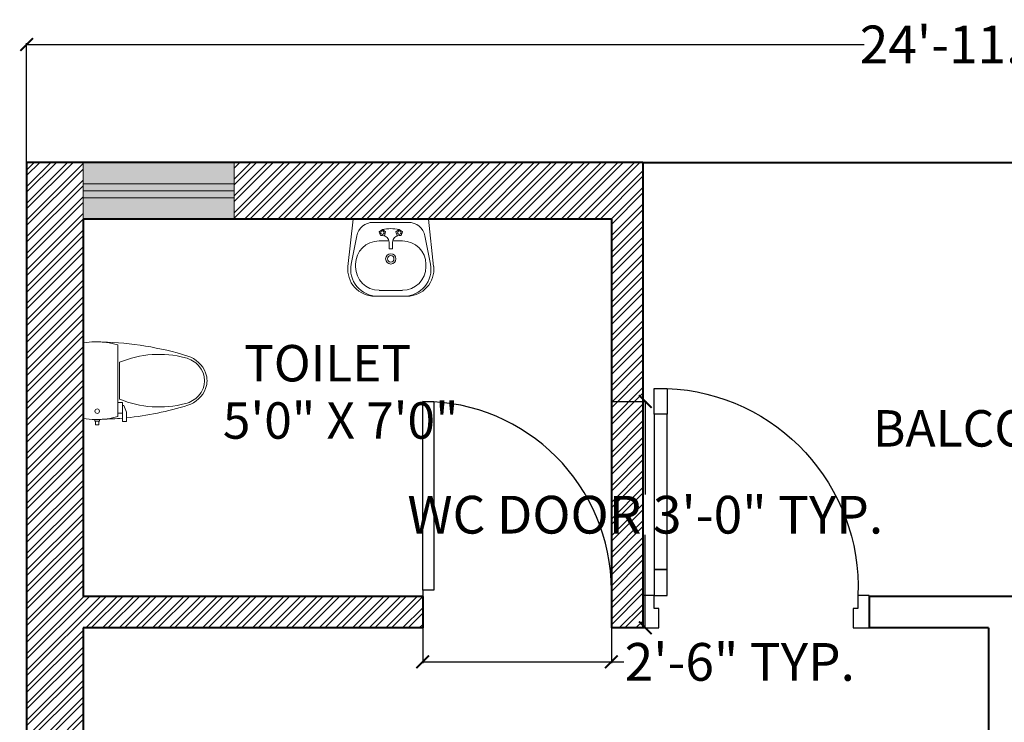
# Model space of a CAD drawing. Units: inches. Extents: x 528 to 2520, y -151 to 1354.
# Tile 20 of 41: x 1123 to 1279, y 1228 to 1340. Entities that reach past the tile are written whole.
import ezdxf

# ---------------------------------------------------------------- set-up
doc = ezdxf.new("R2010")
doc.units = ezdxf.units.IN
doc.header["$MEASUREMENT"] = 0
for name, color, linetype, lineweight in [('A-ANNO-DIMS', 2, 'Continuous', 18), ('A-AREA-IDEN', 7, 'Continuous', 18), ('A-Door', 150, 'Continuous', 25), ('A-FLOR-FIXT', 9, 'Continuous', 18), ('A-WALL-PATT', 6, 'Continuous', 13), ('walls', 7, 'Continuous', 40), ('WINDOWS', 2, 'Continuous', 20)]:
    doc.layers.add(name, color=color, linetype=linetype, lineweight=lineweight)
doc.layers.add('A-GLAZ-PATT', color=152, linetype='Continuous', lineweight=13, true_color=0x2776bb)
doc.layers.add('NT', color=1, linetype='Continuous')
doc.styles.get("Standard").update_dxf_attribs({"font": 'arial.ttf'})
doc.dimstyles.get("Standard").update_dxf_attribs({"dimtxt": 6, "dimasz": 2, "dimexe": 0.18, "dimexo": 0.0625, "dimgap": 0.09, "dimtad": 0, "dimtih": 1, "dimtoh": 1, "dimdec": 1, "dimzin": 0, "dimdsep": 46, "dimlunit": 3, "dimtxsty": 'Standard', "dimblk": 'ARCHTICK', "dimcen": 0.09, "dimadec": 0, "dimazin": 0, "dimtfac": 1, "dimtdec": 1, "dimtofl": 0, "dimtmove": 0, "dimatfit": 3, "dimfxl": 1, "dimtolj": 1, "dimtzin": 0, "dimarcsym": 0})

# ---------------------------------------------------------------- blocks, each defined once
blk = doc.blocks.new('A$C7DB75F4D')
at = {"layer": 'A-Door'}
for points in [[(625, 740), (625, 660), (665, 660), (665, 740)], [(625, 180), (625, 660), (665, 660), (665, 180)], [(625, 100), (625, 180), (665, 180), (665, 100)], [(35, 100), (35, 60), (50, 60), (50, 50), (50, 0), (0, 0), (0, 100)], [(665, 100), (700, 100), (700, 0), (650, 0), (650, 50), (650, 60), (665, 60)]]:
    blk.add_lwpolyline(points, close=True, dxfattribs=at)
at = {"layer": 'NT'}
blk.add_arc((650, 125), 615.5, 92.3278, 182.3278, dxfattribs=at)
blk = doc.blocks.new('toilet-7')
at = {"color": 0, "linetype": 'ByBlock'}
for p, q in [((0.2097, -0.02), (-0.2097, -0.02)), ((0.2151, -0.0677), (0.2097, -0.02)), ((-0.2457, -0.0874), (-0.2457, -0.1068)), ((-0.2457, -0.0874), (-0.2257, -0.0874)), ((-0.2457, -0.1068), (-0.2257, -0.1068)), ((-0.2257, -0.0846), (-0.2257, -0.1096)), ((-0.2257, -0.0846), (-0.2157, -0.0846)), ((0.2151, -0.1171), (0.2151, -0.0677)), ((-0.2257, -0.1096), (-0.2154, -0.1096)), ((0.1991, -0.2124), (0.2099, -0.164)), ((0.2099, -0.164), (0.2151, -0.1171)), ((0.1991, -0.2124), (-0.1991, -0.2124)), ((-0.1803, -0.2374), (-0.1803, -0.2124)), ((-0.1213, -0.2374), (-0.1213, -0.2124)), ((-0.1213, -0.2374), (-0.2278, -0.2374)), ((-0.2278, -0.2374), (-0.2278, -0.2599)), ((-0.1759, -0.2599), (-0.2278, -0.2599)), ((-0.1759, -0.2599), (-0.1379, -0.2451)), ((-0.1379, -0.2451), (-0.1379, -0.2374)), ((-0.1023, -0.2212), (0.1023, -0.2212))]:
    blk.add_line(p, q, dxfattribs=at)
blk.add_circle((-0.1696, -0.0971), 0.0125, dxfattribs=at)
for centre, radius, start, end in [((0.2244, -0.0924), 0.4402, 170.5377, 187.7399), ((1.517, -0.087), 1.7318, 181.2224, 184.9822), ((0.2244, -0.0924), 0.4402, 187.7399, 195.822), ((-1.517, -0.087), 1.7318, 342.7523, 358.7776), ((1.517, -0.087), 1.7318, 185.7323, 197.2477), ((0.4258, -0.4413), 0.5721, 157.3737, 194.7786), ((-0.4258, -0.4413), 0.5721, 345.2214, 22.6263), ((0.0116, -0.5544), 0.1554, 197.2477, 249.5476), ((0.0221, -0.5478), 0.1546, 194.7786, 226.8543), ((-0.0116, -0.5544), 0.1554, 290.4524, 342.7523), ((-0.0221, -0.5478), 0.1546, 313.1457, 345.2214), ((0, -0.5713), 0.1223, 226.8543, 313.1457), ((0, -0.5854), 0.1223, 249.5476, 290.4524)]:
    blk.add_arc(centre, radius, start, end, dxfattribs=at)
blk = doc.blocks.new('_ArchTick')
at = {"color": 0, "linetype": 'ByBlock', "const_width": 0.15}
blk.add_lwpolyline([(-0.5, -0.5), (0.5, 0.5)], dxfattribs=at)
blk = doc.blocks.new('*D27')
at = {"layer": 'A-ANNO-DIMS', "color": 0, "lineweight": -2, "transparency": 16777216}
for p, q in [((1123.88, 1317.17), (1123.88, 1336.05)), ((1123.88, 1335.87), (1257.11, 1335.87)), ((1422.88, 1335.87), (1289.66, 1335.87)), ((1422.88, 1317.17), (1422.88, 1336.05))]:
    blk.add_line(p, q, dxfattribs=at)
at = {"layer": 'Defpoints', "color": 0, "transparency": 16777216}
for p in [(1422.88, 1335.87), (1123.88, 1317.1), (1422.88, 1317.1)]:
    blk.add_point(p, dxfattribs=at)
at = {"layer": 'A-ANNO-DIMS', "color": 0, "lineweight": -2, "transparency": 16777216, "xscale": 2, "yscale": 2, "zscale": 2, "rotation": 180}
blk.add_blockref('_ArchTick', (1123.88, 1335.87), dxfattribs=at)
at = {"layer": 'A-ANNO-DIMS', "color": 0, "lineweight": -2, "transparency": 16777216, "xscale": 2, "yscale": 2, "zscale": 2}
blk.add_blockref('_ArchTick', (1422.88, 1335.87), dxfattribs=at)
at = {"layer": 'A-ANNO-DIMS', "color": 0, "transparency": 16777216, "insert": (1273.38, 1335.87), "char_height": 6, "attachment_point": 5}
blk.add_mtext('\\A1;24\'-11.0"', dxfattribs=at)
blk = doc.blocks.new('BASIN-WITH-TAP')
for p, q in [((0.84, 12.27), (0.02, 4.73)), ((12.84, 12.27), (0.84, 12.27)), ((9.64, 11.73), (4.05, 11.73)), ((12.84, 12.27), (13.66, 4.73)), ((1.43, 9.58), (0.55, 5.09)), ((5, 10.24), (5.51, 10.61)), ((5.2, 9.64), (5, 10.24)), ((5.24, 10.1), (5.2, 10.1)), ((5.24, 9.64), (5.51, 9.64)), ((5.51, 10.61), (6.02, 10.24)), ((6.02, 10.24), (5.82, 9.64)), ((8.18, 10.61), (7.67, 10.24)), ((7.67, 10.24), (7.86, 9.64)), ((8.68, 10.24), (8.18, 10.61)), ((8.49, 9.64), (8.18, 9.64)), ((8.44, 10.1), (8.49, 10.1)), ((8.49, 9.64), (8.68, 10.24)), ((12.26, 9.58), (13.14, 5.09)), ((4.98, 8.8), (6.58, 8.8)), ((6.58, 8.31), (6.58, 8.58)), ((6.58, 7.51), (6.58, 8.31)), ((8.71, 8.8), (7.11, 8.8)), ((7.11, 8.31), (7.11, 8.58)), ((7.11, 7.51), (7.11, 8.31)), ((6.58, 7.51), (7.11, 7.51)), ((1.24, 4.67), (1.24, 5.07)), ((12.44, 4.67), (12.44, 5.07)), ((4.73, 0), (8.96, 0)), ((6.84, 0.93), (4.98, 0.93)), ((6.84, 0.93), (8.71, 0.93))]:
    blk.add_line(p, q)
for centre, radius in [((5.5, 10.1), 0.277), ((8.19, 10.1), 0.277), ((6.84, 5.94), 0.821), ((6.84, 5.94), 0.507)]:
    blk.add_circle(centre, radius)
for centre, radius, start, end in [((4.05, 9.07), 2.67, 90, 168.8773), ((9.64, 9.07), 2.67, 11.1227, 90), ((6.84, 4.01), 6.73, 78.5788, 101.4212), ((5.51, 8.58), 1.07, 0, 90), ((8.18, 8.58), 1.07, 90, 180), ((4.98, 5.07), 3.73, 90, 180), ((8.71, 5.07), 3.73, 0, 90), ((4.27, 4.27), 4.27, 173.7966, 270), ((4.73, 4.27), 4.27, 168.8773, 270), ((8.96, 4.27), 4.27, 270, 11.1227), ((9.42, 4.27), 4.27, 270, 6.2034), ((4.98, 4.67), 3.73, 180, 270), ((8.71, 4.67), 3.73, 270, 0)]:
    blk.add_arc(centre, radius, start, end)
blk = doc.blocks.new('DOOR-SWING-30')
for p, q in [((0, 6), (0, 0)), ((30, 6), (30, 0))]:
    blk.add_line(p, q)
blk.add_lwpolyline([(0, 6), (0, 36), (1.75, 36), (1.75, 6)], close=True)
blk.add_arc((0, 6), 30, 0, 90)
blk = doc.blocks.new('WINDOW-24x9-PLAN')
for p, q in [((0, 5.63), (24, 5.63)), ((0, 4.5), (24, 4.5)), ((0, 3.37), (24, 3.37))]:
    blk.add_line(p, q)
blk.add_lwpolyline([(0, 9), (24, 9), (24, 0), (0, 0)], close=True)
blk = doc.blocks.new('*D54')
at = {"layer": 'A-ANNO-DIMS', "color": 0, "lineweight": -2, "transparency": 16777216}
for p, q in [((1216.95, 1279.1), (1222.46, 1279.1)), ((1222.28, 1279.1), (1222.28, 1264.3)), ((1222.28, 1243.1), (1222.28, 1257.91)), ((1216.95, 1243.1), (1222.46, 1243.1))]:
    blk.add_line(p, q, dxfattribs=at)
at = {"layer": 'Defpoints', "color": 0, "transparency": 16777216}
for p in [(1216.88, 1279.1), (1222.28, 1279.1), (1216.88, 1243.1)]:
    blk.add_point(p, dxfattribs=at)
at = {"layer": 'A-ANNO-DIMS', "color": 0, "lineweight": -2, "transparency": 16777216, "xscale": 2, "yscale": 2, "zscale": 2}
for p, rotation in [((1222.28, 1279.1), 90), ((1222.28, 1243.1), 270)]:
    blk.add_blockref('_ArchTick', p, dxfattribs=dict(at, rotation=rotation))
at = {"layer": 'A-ANNO-DIMS', "color": 0, "transparency": 16777216, "insert": (1222.28, 1261.1), "char_height": 6, "attachment_point": 5}
blk.add_mtext('\\A1;WC DOOR 3\'-0" TYP.', dxfattribs=at)
blk = doc.blocks.new('*D55')
at = {"layer": 'A-ANNO-DIMS', "color": 0, "lineweight": -2, "transparency": 16777216}
for p, q in [((1186.88, 1243.04), (1186.88, 1237.52)), ((1216.88, 1243.04), (1216.88, 1237.52)), ((1186.88, 1237.7), (1216.88, 1237.7)), ((1216.88, 1237.7), (1218.88, 1237.7))]:
    blk.add_line(p, q, dxfattribs=at)
at = {"layer": 'Defpoints', "color": 0, "transparency": 16777216}
for p in [(1186.88, 1243.1), (1216.88, 1243.1), (1216.88, 1237.7)]:
    blk.add_point(p, dxfattribs=at)
at = {"layer": 'A-ANNO-DIMS', "color": 0, "lineweight": -2, "transparency": 16777216, "xscale": 2, "yscale": 2, "zscale": 2, "rotation": 180}
blk.add_blockref('_ArchTick', (1186.88, 1237.7), dxfattribs=at)
at = {"layer": 'A-ANNO-DIMS', "color": 0, "lineweight": -2, "transparency": 16777216, "xscale": 2, "yscale": 2, "zscale": 2}
blk.add_blockref('_ArchTick', (1216.88, 1237.7), dxfattribs=at)
at = {"layer": 'A-ANNO-DIMS', "color": 0, "transparency": 16777216, "insert": (1237.31, 1237.7), "char_height": 6, "attachment_point": 5}
blk.add_mtext('\\A1;2\'-6" TYP.', dxfattribs=at)

msp = doc.modelspace()

# ---------------------------------------------------------------- hatches: boundary and pattern name
at = {"layer": 'A-GLAZ-PATT'}
h = msp.add_hatch(color=256, dxfattribs=at)
h.dxf.hatch_style = 1
h.paths.add_polyline_path([(1156.88, 1313.73), (1132.88, 1313.73), (1132.88, 1312.6), (1156.88, 1312.6)])
h.paths.add_polyline_path([(1156.88, 1312.6), (1132.88, 1312.6), (1132.88, 1311.47), (1156.88, 1311.47)])
h.paths.add_polyline_path([(1156.88, 1317.1), (1132.88, 1317.1), (1132.88, 1313.73), (1156.88, 1313.73)])
h.paths.add_polyline_path([(1156.88, 1311.47), (1132.88, 1311.47), (1132.88, 1308.1), (1156.88, 1308.1)])
at = {"layer": 'A-WALL-PATT'}
h = msp.add_hatch(dxfattribs=at)
h.set_pattern_fill('ANSI32', color=256, scale=5)
h.set_pattern_definition([(45, (537.1868, 0), (-1.3258252, 1.3258252), []), (45, (538.0707, 0), (-1.3258252, 1.3258252), [])])
h.paths.add_polyline_path([(1132.88, 1163.86), (1123.88, 1163.86), (1123.88, 969.1), (1135.43, 969.1), (1140.43, 969.1), (1140.43, 974.1), (1132.88, 974.1), (1132.88, 1082.1), (1228.88, 1082.1), (1228.88, 1087.1), (1228.88, 1106.1), (1234.88, 1106.1), (1234.88, 1111.1), (1223.88, 1111.1), (1223.88, 1087.1), (1132.88, 1087.1)])
h.paths.add_polyline_path([(1225.89, 974.1), (1188.43, 974.1), (1188.43, 969.1), (1225.89, 969.1)])
h.paths.add_polyline_path([(1422.88, 1171.37), (1413.88, 1171.37), (1413.88, 1111.1), (1323.88, 1111.1), (1323.88, 1106.1), (1413.88, 1106.1), (1413.88, 974.1), (1323.88, 974.1), (1323.88, 969.1), (1413.88, 969.1), (1413.88, 825.1), (1371.88, 825.1), (1371.88, 816.1), (1422.88, 816.1)])
h.paths.add_polyline_path([(1422.88, 1317.1), (1413.84, 1317.1), (1413.84, 1308.1), (1413.88, 1308.1), (1413.88, 1248.1), (1359.88, 1248.1), (1359.88, 1243.1), (1413.88, 1243.1), (1413.88, 1219.37), (1422.88, 1219.37)])
h.paths.add_polyline_path([(1389.84, 1317.1), (1324.88, 1317.1), (1324.88, 1248.1), (1321.45, 1248.1), (1321.45, 1243.1), (1329.88, 1243.1), (1329.88, 1249.1), (1329.88, 1308.1), (1389.84, 1308.1)])
h.paths.add_polyline_path([(1221.88, 1317.1), (1156.88, 1317.1), (1156.88, 1308.1), (1216.88, 1308.1), (1216.88, 1248.1), (1216.88, 1243.1), (1221.88, 1243.1), (1221.88, 1248.25)])
h.paths.add_polyline_path([(1132.88, 1308.1), (1132.88, 1317.1), (1123.88, 1317.1), (1123.88, 1211.86), (1132.88, 1211.86), (1132.88, 1243.1), (1186.88, 1243.1), (1186.88, 1248.1), (1132.88, 1248.1)])
h.paths.add_polyline_path([(1281.88, 969.1), (1281.88, 974.1), (1261.89, 974.1), (1261.89, 969.1), (1276.88, 969.1), (1276.88, 874.29), (1281.88, 874.29)])
h.paths.add_polyline_path([(1276.88, 969.1), (1264.88, 969.1), (1264.88, 965.12), (1267.92, 965.12), (1267.92, 961.68), (1271.62, 961.68), (1271.62, 957.24), (1276.88, 957.24)], flags=17)
h.paths.add_polyline_path([(1323.88, 825.1), (1281.88, 825.1), (1281.88, 832.29), (1276.88, 832.29), (1276.88, 816.1), (1323.88, 816.1)])

# ---------------------------------------------------------------- linework, layer by layer
at = {"layer": 'walls'}
for p, q in [((1123.88, 1317.1), (1123.88, 969.1)), ((1221.88, 1317.1), (1123.88, 1317.1)), ((1221.88, 1317.1), (1221.88, 1248.1)), ((1221.88, 1317.1), (1324.88, 1317.1)), ((1132.88, 1308.1), (1132.88, 1248.1)), ((1216.88, 1308.1), (1132.88, 1308.1)), ((1216.88, 1308.1), (1216.88, 1248.1)), ((1186.88, 1248.1), (1132.88, 1248.1)), ((1186.88, 1248.1), (1186.88, 1243.1)), ((1216.88, 1248.1), (1216.88, 1243.1)), ((1221.88, 1248.1), (1221.88, 1243.1)), ((1324.88, 1248.1), (1257.88, 1248.1)), ((1257.88, 1248.1), (1257.88, 1243.1)), ((1132.88, 1243.1), (1132.88, 1087.1)), ((1186.88, 1243.1), (1132.88, 1243.1)), ((1221.88, 1243.1), (1216.88, 1243.1)), ((1276.88, 1243.1), (1257.88, 1243.1)), ((1276.88, 1243.1), (1276.88, 1111.1))]:
    msp.add_line(p, q, dxfattribs=at)

# ---------------------------------------------------------------- block references
at = {"layer": 'A-Door', "xscale": -0.0514539602427209, "yscale": 0.0514539602427209, "zscale": 0.0514539602427209}
msp.add_blockref('A$C7DB75F4D', (1257.9, 1243.1), dxfattribs=at)
at = {"layer": 'A-Door'}
msp.add_blockref('DOOR-SWING-30', (1186.88, 1243.1), dxfattribs=at)
at = {"layer": 'A-FLOR-FIXT'}
msp.add_blockref('BASIN-WITH-TAP', (1174.96, 1295.84), dxfattribs=at)
at = {"layer": 'A-FLOR-FIXT', "xscale": 28.60654769571749, "yscale": 28.60654769571749, "zscale": 28.60654769571749, "rotation": 90}
msp.add_blockref('toilet-7', (1132.33, 1282.41), dxfattribs=at)
at = {"layer": 'WINDOWS'}
msp.add_blockref('WINDOW-24x9-PLAN', (1132.88, 1308.1), dxfattribs=at)

# ---------------------------------------------------------------- texts
at = {"layer": 'A-AREA-IDEN'}
for s, height, p in [('TOILET', 5.793, (1158.46, 1282.29)), ('5\'0" X 7\'0"', 5.7926, (1155.09, 1273.18)), ('BALCONY', 5.793, (1258.47, 1271.93))]:
    msp.add_text(s, height=height, dxfattribs=at).set_placement(p)

# ---------------------------------------------------------------- dimensions: what is measured, and where the dimension line sits
at = {"layer": 'A-ANNO-DIMS'}
dim = msp.add_linear_dim(base=(1422.88, 1335.87), p1=(1123.88, 1317.1), p2=(1422.88, 1317.1), dimstyle='Standard', override={"dimclrd": 0, "dimclre": 0, "dimclrt": 0}, dxfattribs=at)
dim.commit()
dim.dimension.update_dxf_attribs({"geometry": '*D27', "text_midpoint": (1273.38, 1335.87)})
dim = msp.add_linear_dim(base=(1222.28, 1279.1), p1=(1216.88, 1243.1), p2=(1216.88, 1279.1), angle=90, text='WC DOOR <> TYP.', dimstyle='Standard', override={"dimdec": 1, "dimlfac": 1, "dimrnd": 0, "dimzin": 1, "dimdsep": 46, "dimlunit": 4, "dimfrac": 2}, dxfattribs=at)
dim.commit()
dim.dimension.update_dxf_attribs({"geometry": '*D54', "text_midpoint": (1222.28, 1261.1)})
dim = msp.add_linear_dim(base=(1216.88, 1237.7), p1=(1186.88, 1243.1), p2=(1216.88, 1243.1), text='<> TYP.', dimstyle='Standard', override={"dimdec": 1, "dimlfac": 1, "dimrnd": 0, "dimzin": 1, "dimdsep": 46, "dimlunit": 4, "dimfrac": 2}, dxfattribs=at)
dim.commit()
dim.dimension.update_dxf_attribs({"geometry": '*D55', "text_midpoint": (1237.31, 1237.7)})

doc.saveas('drawing.dxf')
